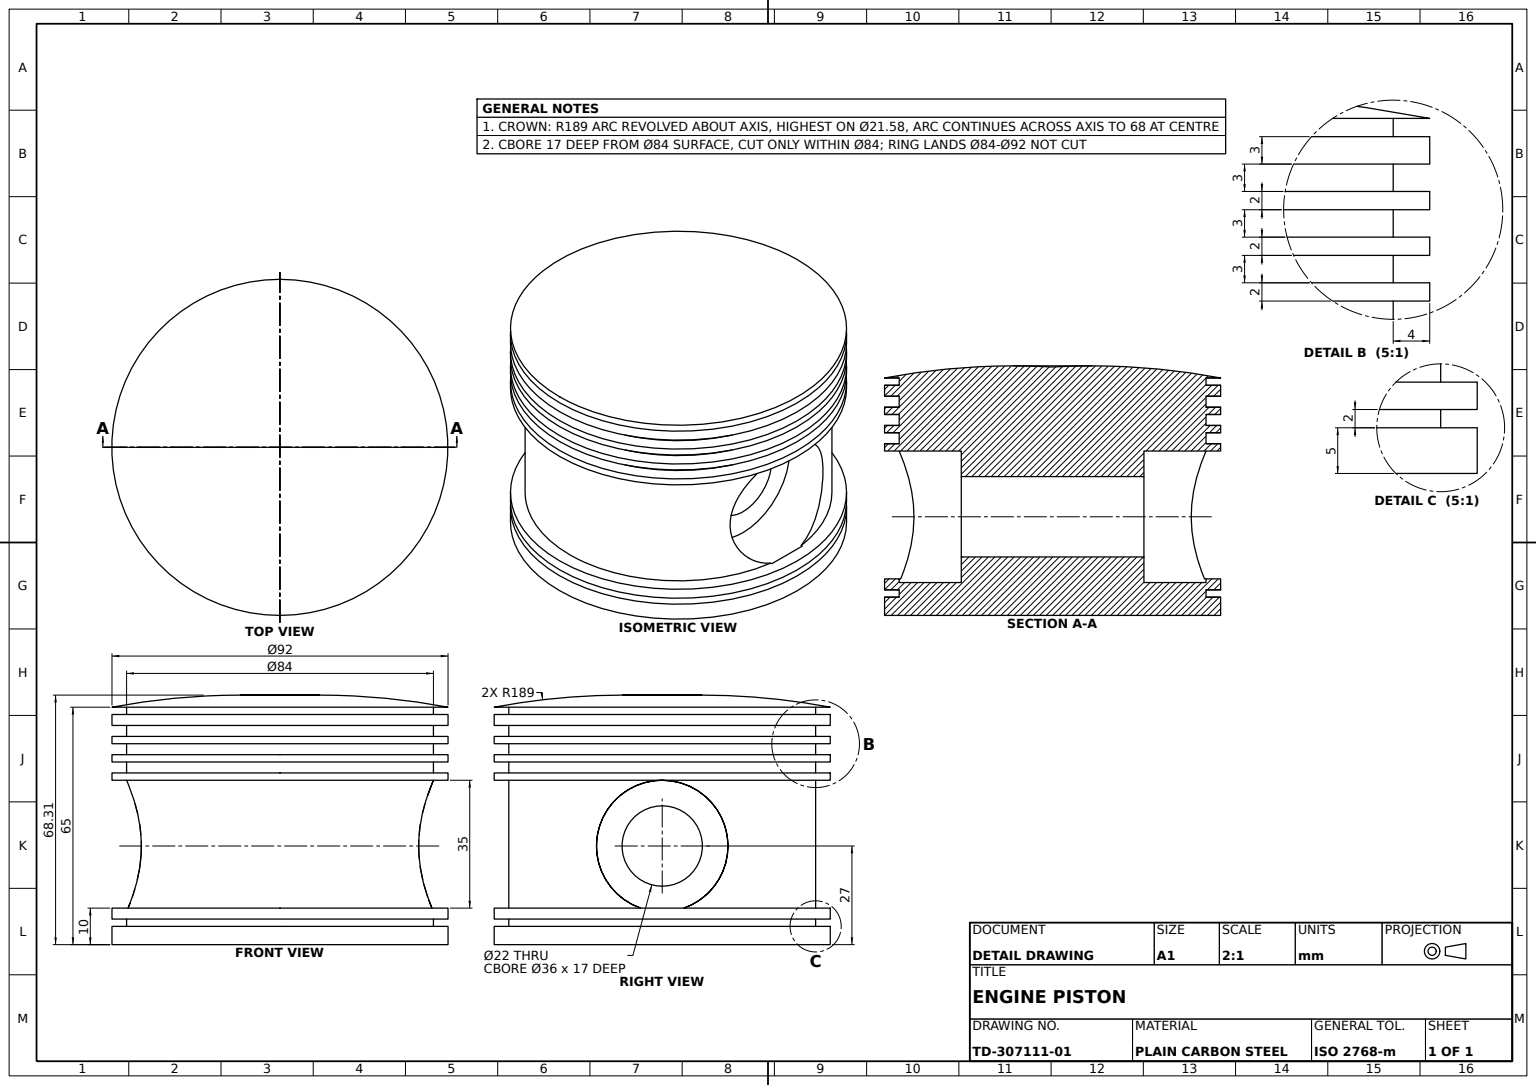
from build123d import *

# Parameters (mm, degrees)
PIN_BOSS_RELIEF_SKETCH_R = 18
PIN_BOSS_RELIEF_36_DEPTH = 17
WRIST_PIN_BORE_SKETCH_R  = 11
WRIST_PIN_BORE_DEPTH     = 157


with BuildPart() as part:
    # Piston Profile Sketch → Piston Body (revolve)
    with BuildSketch(Plane(origin=(0, 0, 0), x_dir=(1, 0, 0), z_dir=(0, 1, 0))):
        with BuildLine():
            ThreePointArc((0, 68), (23.091806354, 67.907697429), (46, 65))
            Line((46, 65), (42, 65))
            Line((42, 65), (42, 63))
            Line((42, 63), (46, 63))
            Line((46, 63), (46, 60))
            Line((46, 60), (42, 60))
            Line((42, 60), (42, 57))
            Line((42, 57), (46, 57))
            Line((46, 57), (46, 55))
            Line((46, 55), (42, 55))
            Line((42, 55), (42, 52))
            Line((42, 52), (46, 52))
            Line((46, 52), (46, 50))
            Line((46, 50), (42, 50))
            Line((42, 50), (42, 47))
            Line((42, 47), (46, 47))
            Line((46, 47), (46, 45))
            Line((46, 45), (42, 45))
            Line((42, 45), (42, 10.377701479))
            Line((42, 10.377701479), (42, 10))
            Line((42, 10), (46, 10))
            Line((46, 10), (46, 7))
            Line((46, 7), (42, 7))
            Line((42, 7), (42, 5))
            Line((42, 5), (46, 5))
            Line((46, 5), (46, 0))
            Line((46, 0), (0, 0))
            Line((0, 0), (0, 68))
        make_face()
    revolve(axis=Axis((0, 0, 0), (0, 0, -1)))

    # Pin Boss Relief Sketch → Pin Boss Relief Ø36 (cut)
    with BuildSketch(Plane(origin=(0, 42, 0), x_dir=(1, 0, 0), z_dir=(0, 1, 0))):
        with Locations(Location((0, 27, 0), (0, 0, 270))):
            Circle(PIN_BOSS_RELIEF_SKETCH_R)
    pin_boss_relief_36 = extrude(amount=-PIN_BOSS_RELIEF_36_DEPTH, mode=Mode.SUBTRACT)

    # Pin Boss Relief Mirror: Pin Boss Relief Ø36 across plane
    add(pin_boss_relief_36.mirror(Plane.ZX), mode=Mode.SUBTRACT)

    # Wrist Pin Bore Sketch → Wrist Pin Bore (cut)
    with BuildSketch(Plane(origin=(0, 25, 0), x_dir=(1, 0, 0), z_dir=(0, 1, 0))):
        with Locations(Location((0, 27, 0), (0, 0, 270))):
            Circle(WRIST_PIN_BORE_SKETCH_R)
    extrude(amount=-WRIST_PIN_BORE_DEPTH, mode=Mode.SUBTRACT)


solid = part.part
